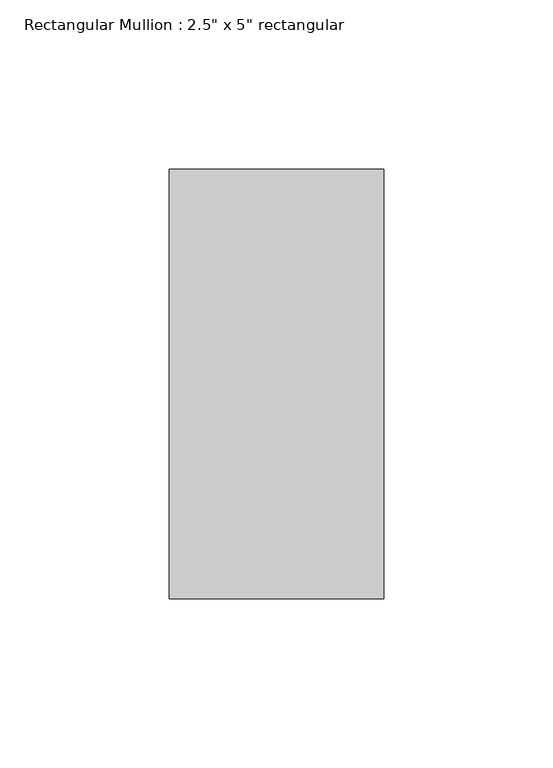
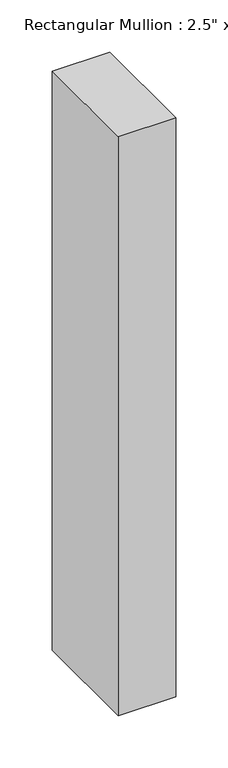
"""IFC4 building model written with IfcOpenShell, lengths in millimetres: member geometry."""

from ifc_helpers import new_model, si_unit, frame, origin, place, context, project, spatial, polyline, outline, extrude, source, transform, mapped, element, save


def member_26d576e8(model_context):
    return source(origin(), model_context, "Body", "SweptSolid", [
        extrude(outline(polyline([(0.0, 63.5), (0.0, -63.5), (-63.5, -63.5), (-63.5, 63.5), (0.0, 63.5)])), frame((0.0, 0.0, -677.3333333), z_axis=(0.0, 0.0, 1.0), x_axis=(1.0, 0.0, 0.0)), (0.0, 0.0, 1.0), 677.3333333),
    ])


if __name__ == "__main__":
    model = new_model("IFC4")
    model_context = context("Model", 3, world=origin())
    ifc_project = project(units=[si_unit("LENGTHUNIT", "METRE", prefix="MILLI")], contexts=[model_context])
    site = spatial("IfcSite", under=ifc_project)
    building = spatial("IfcBuilding", under=site)
    placement = place(None, origin())
    member_shape = member_26d576e8(model_context)
    element("IfcMember", 1, ObjectType="Rectangular Mullion : 2.5\" x 5\" rectangular", at=placement, inside=building, context=model_context, shape_type="MappedRepresentation", body=[
        mapped(member_shape, transform((0.0, 0.0, 0.0), x_axis=(1.0, 0.0, 0.0), y_axis=(0.0, 1.0, 0.0), z_axis=(0.0, 0.0, 1.0))),
    ])
    save(model, "model.ifc")

# Revit data of these elements
# Type "Rectangular Mullion : 2.5\" x 5\" rectangular"
#   built-in parameter 1007304 = 0.416667 (stored number, unit not read)
#   built-in parameter 1007301 = 0.104167 (stored number, unit not read)
#   built-in parameter 1007300 = 0.104167 (stored number, unit not read)
# Element 1 (IfcMember, "Rectangular Mullion : 2.5\" x 5\" rectangular")
#   Materials on its faces: "door colour"
# Materials
#   "door colour": class "Generic", colour RGB 120 120 120, transparency 0, Cost = 0
